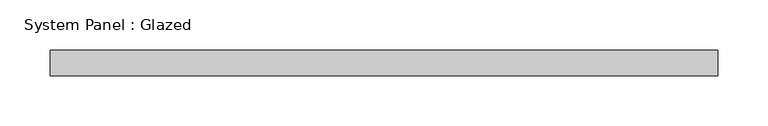
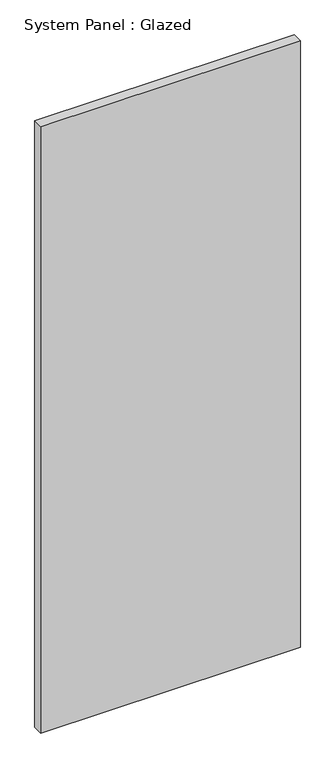
"""IFC4 building model written with IfcOpenShell, lengths in millimetres: plate geometry, System Panel : Glazed."""

from ifc_helpers import new_model, si_unit, origin, origin_with_axes, place, context, project, spatial, polyline, outline, extrude, source, transform, mapped, element, save


def system_panel_glazed_7f229d02(model_context):
    return source(origin(), model_context, "Body", "SweptSolid", [
        extrude(outline(polyline([(333.375, 19.05), (-333.375, 19.05), (-333.375, 44.45), (333.375, 44.45), (333.375, 19.05)])), origin_with_axes(), (0.0, 0.0, 1.0), 1644.500021),
    ])


if __name__ == "__main__":
    model = new_model("IFC4")
    model_context = context("Model", 3, world=origin())
    ifc_project = project(units=[si_unit("LENGTHUNIT", "METRE", prefix="MILLI")], contexts=[model_context])
    site = spatial("IfcSite", under=ifc_project)
    building = spatial("IfcBuilding", under=site)
    placement = place(None, origin())
    system_panel_glazed_shape = system_panel_glazed_7f229d02(model_context)
    element("IfcPlate", 1, ObjectType="System Panel : Glazed", at=placement, inside=building, context=model_context, shape_type="MappedRepresentation", body=[
        mapped(system_panel_glazed_shape, transform((0.0, 0.0, 0.0), x_axis=(1.0, 0.0, 0.0), y_axis=(0.0, 1.0, 0.0), z_axis=(0.0, 0.0, 1.0))),
    ])
    save(model, "model.ifc")

# Revit data of these elements
# Type "System Panel : Glazed"
#   Construction Type Id = "GSP4R"
#   Analytic Construction = "1/8 in Pilkington single glazing"
#   Visual Light Transmittance = 0.9
#   Solar Heat Gain Coefficient = 0.86
#   Heat Transfer Coefficient (U) = 1.18115 BTU/(h·ft²·°F)
#   Define Thermal Properties by = 1
# Element 1 (IfcPlate, "System Panel : Glazed")
#   Materials on its faces: "Glass"
# Materials
#   "Glass": class "Glass", colour RGB 0 128 192, transparency 0.75, Description = "Soda Lime Glass", Cost = 0
